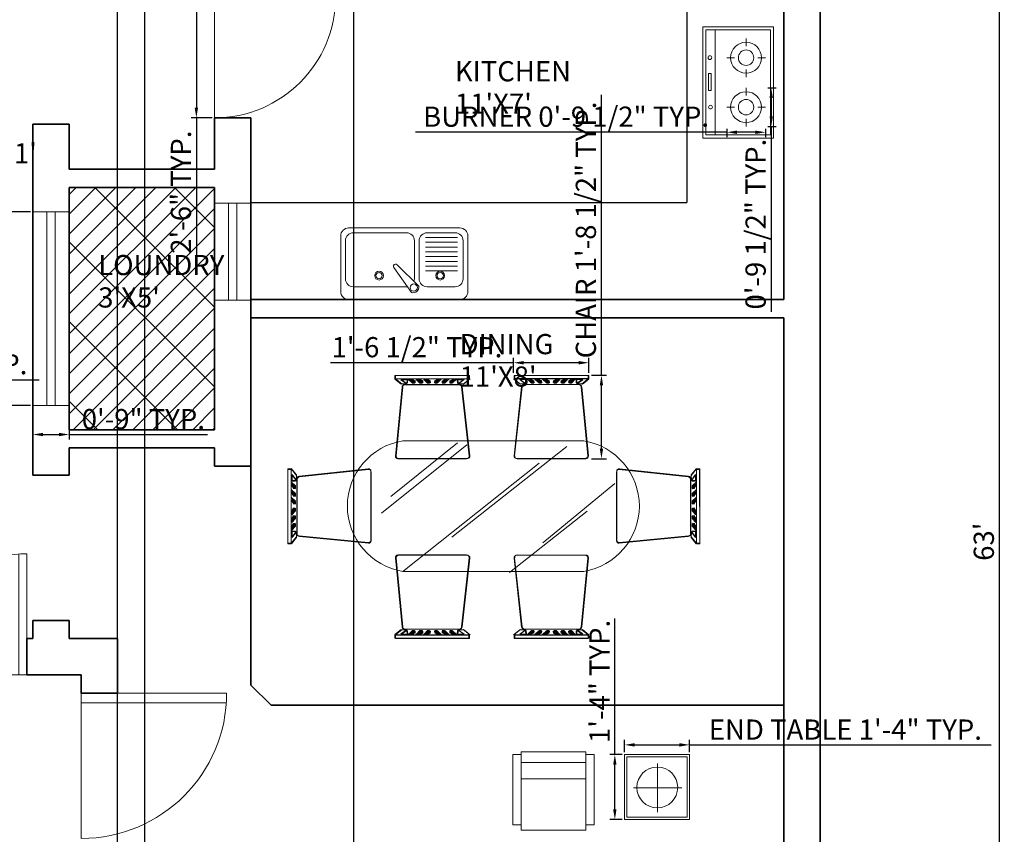
# Model space of a CAD drawing. Units: inches. Extents: x 1265 to 2734, y 1741 to 2595.
# Tile 7 of 10: x 2490 to 2734, y 2092 to 2294. Entities that reach past the tile are written whole.
import ezdxf

# ---------------------------------------------------------------- set-up
doc = ezdxf.new("R2010")
doc.units = ezdxf.units.IN
doc.header["$LTSCALE"] = 0.1
for name, color, linetype, lineweight in [('A-ANNO-DIMS', 2, 'Continuous', 18), ('A-ANNO-TEXT', 7, 'Continuous', 18), ('A-AREA-IDEN', 7, 'Continuous', 18), ('A-DOOR', 3, 'Continuous', 18), ('A-EQPM', 9, 'Continuous', 18), ('A-FLOR-CASE', 33, 'Continuous', 25), ('A-FLOR-FIXT', 9, 'Continuous', 18), ('A-FLOR-PATT', 252, 'Continuous', 13), ('A-GLAZ', 4, 'Continuous', 18), ('A-WALL', 7, 'Continuous', 35), ('C-PROP', 7, 'Continuous', 35), ('Furniture', 8, 'Continuous', 15)]:
    doc.layers.add(name, color=color, linetype=linetype, lineweight=lineweight)
doc.styles.get("Standard").update_dxf_attribs({"font": 'arial.ttf', "height": 5})
doc.dimstyles.new('ISO-25', dxfattribs={"dimtxt": 5, "dimasz": 2.5, "dimexe": 1.25, "dimexo": 0.625, "dimtad": 1, "dimlunit": 3, "dimtxsty": 'Standard', "dimcen": 2.5, "dimadec": 0, "dimazin": 0, "dimtfac": 1, "dimtmove": 0, "dimatfit": 3, "dimfxl": 1, "dimarcsym": 0})

# ---------------------------------------------------------------- blocks, each defined once
blk = doc.blocks.new('*D3')
at = {"layer": 'A-ANNO-DIMS', "color": 0, "lineweight": -2, "transparency": 16777216}
for p, q in [((2689.23, 2542.66), (2734.23, 2542.66)), ((2732.98, 2540.16), (2732.98, 1789.16)), ((2689.23, 1786.66), (2734.23, 1786.66))]:
    blk.add_line(p, q, dxfattribs=at)
at = {"layer": 'A-ANNO-DIMS', "color": 0, "lineweight": 100, "transparency": 16777216}
for points in [[(2732.56, 2540.16), (2733.39, 2540.16), (2732.98, 2542.66)], [(2732.56, 1789.16), (2733.39, 1789.16), (2732.98, 1786.66)]]:
    blk.add_solid(points, dxfattribs=at)
at = {"layer": 'Defpoints', "color": 0, "lineweight": 100, "transparency": 16777216}
for p in [(2688.6, 2542.66), (2688.6, 1786.66), (2732.98, 1786.66)]:
    blk.add_point(p, dxfattribs=at)
at = {"layer": 'A-ANNO-DIMS', "color": 0, "transparency": 16777216, "insert": (2729.8, 2164.66), "char_height": 5, "attachment_point": 5, "rotation": 90}
blk.add_mtext("63'", dxfattribs=at)
blk = doc.blocks.new('DOOR-SWING-30IN')
for p, q in [((30, 0), (30, 30)), ((0.07, 2), (30, 2)), ((0, 0), (30, 0))]:
    blk.add_line(p, q)
blk.add_arc((30, 0), 30, 90, 180)
blk = doc.blocks.new('DOOR-SWING-36IN')
for p, q in [((33.6, 35.92), (33.6, 0)), ((36, 36), (36, 0)), ((36, 0), (0, 0))]:
    blk.add_line(p, q)
blk.add_arc((36, 0), 36, 90, 180)
blk = doc.blocks.new('DOOR-PAIR-60IN')
for p, q in [((0, 30), (0, 0)), ((2, 29.93), (2, 0)), ((58, 29.93), (58, 0)), ((60, 30), (60, 0)), ((0, 0), (30, 0)), ((60, 0), (30, 0))]:
    blk.add_line(p, q)
for centre, start, end in [((0, 0), 0, 90), ((60, 0), 90, 180)]:
    blk.add_arc(centre, 30, start, end)
blk = doc.blocks.new('WINDOW-24IN')
for p, q in [((9, 24), (0, 24)), ((0, 24), (0, 0)), ((3.5, 24), (3.5, 0)), ((5.5, 24), (5.5, 0)), ((9, 24), (9, 0)), ((9, 0), (0, 0))]:
    blk.add_line(p, q)
blk = doc.blocks.new('WINDOW-48IN')
for p, q in [((0, 9), (0, 0)), ((48, 9), (0, 9)), ((48, 9), (48, 0)), ((48, 5.5), (0, 5.5)), ((48, 3.5), (0, 3.5)), ((0, 0), (48, 0))]:
    blk.add_line(p, q)
blk = doc.blocks.new('CHAIR-DINING')
for p, q in [((0.02, 0.74), (0, 17.76)), ((0.07, 0.9), (0.06, 17.92)), ((0.7, 18.39), (17.79, 16.53)), ((0.76, 18.55), (17.84, 16.69)), ((19.73, 18.48), (18.47, 16.91)), ((19.79, 18.64), (18.53, 17.07)), ((18.59, 15.75), (19.6, 17.13)), ((19.6, 17.13), (19.66, 15.62)), ((20.61, 18.35), (19.79, 18.35)), ((19.79, 18.35), (19.8, 0)), ((20.66, 18.52), (19.85, 18.52)), ((19.85, 18.52), (19.86, 0.16)), ((20.62, 0), (20.61, 18.35)), ((20.68, 0.16), (20.66, 18.52)), ((18.35, 15.9), (18.36, 2.39)), ((18.41, 16.07), (18.42, 2.55)), ((18.47, 16.91), (18.53, 15.59)), ((18.53, 17.07), (18.59, 15.75)), ((18.53, 15.59), (19.54, 16.97)), ((19.6, 15.46), (18.72, 15.52)), ((19.67, 15.09), (18.72, 14.14)), ((19.66, 15.62), (18.78, 15.69)), ((19.73, 15.25), (18.78, 14.3)), ((18.78, 13.8), (19.66, 14.74)), ((19.54, 16.97), (19.6, 15.46)), ((19.66, 14.74), (19.66, 14.37)), ((18.72, 13.64), (19.6, 14.58)), ((18.72, 14.14), (18.72, 13.64)), ((19.67, 13.2), (18.73, 12.26)), ((18.73, 11.75), (19.61, 12.7)), ((18.73, 12.26), (18.73, 11.75)), ((18.78, 14.3), (18.78, 13.8)), ((19.35, 13.64), (18.79, 13.58)), ((19.73, 13.36), (18.79, 12.42)), ((18.79, 11.92), (19.66, 12.86)), ((18.79, 12.42), (18.79, 11.92)), ((19.41, 13.8), (18.85, 13.74)), ((19.6, 14.21), (19.23, 13.76)), ((19.23, 13.76), (19.35, 13.64)), ((19.61, 12.32), (19.23, 11.88)), ((19.66, 14.37), (19.29, 13.93)), ((19.29, 13.93), (19.41, 13.8)), ((19.67, 12.48), (19.29, 12.04)), ((19.6, 14.58), (19.6, 14.21)), ((19.61, 12.7), (19.61, 12.32)), ((19.66, 12.86), (19.67, 12.48)), ((19.67, 11.31), (18.73, 10.37)), ((18.73, 9.87), (19.61, 10.81)), ((18.73, 10.37), (18.73, 9.87)), ((19.35, 11.75), (18.79, 11.69)), ((19.73, 11.48), (18.79, 10.53)), ((18.79, 10.03), (19.67, 10.97)), ((18.79, 10.53), (18.79, 10.03)), ((19.36, 9.87), (18.79, 9.8)), ((19.41, 11.92), (18.85, 11.85)), ((19.42, 10.03), (18.85, 9.97)), ((19.23, 11.88), (19.35, 11.75)), ((19.61, 10.43), (19.23, 9.99)), ((19.23, 9.99), (19.36, 9.87)), ((19.29, 12.04), (19.41, 11.92)), ((19.67, 10.6), (19.29, 10.16)), ((19.29, 10.16), (19.42, 10.03)), ((19.61, 10.81), (19.61, 10.43)), ((19.67, 10.97), (19.67, 10.6)), ((18.73, 8.11), (18.73, 8.61)), ((18.73, 8.61), (19.61, 7.67)), ((19.67, 7.17), (18.73, 8.11)), ((18.79, 8.27), (18.79, 8.77)), ((18.79, 8.77), (19.67, 7.83)), ((19.36, 8.61), (18.79, 8.67)), ((19.73, 7.33), (18.79, 8.27)), ((19.42, 8.77), (18.85, 8.84)), ((19.23, 8.48), (19.36, 8.61)), ((19.61, 8.05), (19.23, 8.48)), ((19.29, 8.65), (19.42, 8.77)), ((19.67, 8.21), (19.29, 8.65)), ((19.61, 7.67), (19.61, 8.05)), ((19.67, 7.83), (19.67, 8.21)), ((18.73, 6.22), (18.73, 6.72)), ((18.73, 6.72), (19.61, 5.78)), ((19.67, 5.28), (18.73, 6.22)), ((18.79, 6.38), (18.79, 6.89)), ((18.79, 6.89), (19.67, 5.94)), ((19.36, 6.73), (18.79, 6.79)), ((19.73, 5.44), (18.79, 6.38)), ((18.79, 4.5), (18.79, 5)), ((18.79, 5), (19.67, 4.06)), ((19.36, 4.84), (18.8, 4.9)), ((19.42, 6.89), (18.85, 6.95)), ((19.42, 5), (18.85, 5.06)), ((19.23, 6.6), (19.36, 6.73)), ((19.61, 6.16), (19.23, 6.6)), ((19.29, 6.76), (19.42, 6.89)), ((19.67, 6.32), (19.29, 6.76)), ((19.29, 4.88), (19.42, 5)), ((19.61, 5.78), (19.61, 6.16)), ((19.67, 5.94), (19.67, 6.32)), ((18.48, 1.57), (18.55, 2.89)), ((18.54, 1.73), (18.61, 3.05)), ((18.55, 2.89), (19.55, 1.51)), ((18.61, 3.05), (19.61, 1.67)), ((18.73, 4.34), (18.73, 4.84)), ((18.73, 4.84), (19.61, 3.9)), ((19.68, 3.39), (18.73, 4.34)), ((19.61, 3.02), (18.73, 2.95)), ((19.74, 3.56), (18.79, 4.5)), ((19.67, 3.18), (18.79, 3.12)), ((19.24, 4.71), (19.36, 4.84)), ((19.61, 4.27), (19.24, 4.71)), ((19.67, 4.44), (19.29, 4.88)), ((19.55, 1.51), (19.61, 3.02)), ((19.61, 3.9), (19.61, 4.27)), ((19.61, 1.67), (19.67, 3.18)), ((19.67, 4.06), (19.67, 4.44)), ((17.79, 1.77), (0.7, 0.11)), ((17.85, 1.93), (0.76, 0.27)), ((19.74, 0), (18.48, 1.57)), ((19.8, 0.16), (18.54, 1.73)), ((19.8, 0), (20.62, 0)), ((19.86, 0.16), (20.68, 0.16))]:
    blk.add_line(p, q)
for centre, start, end in [((0.63, 17.76), 83.7931, 180.0502), ((0.69, 17.92), 83.7931, 180.0502), ((17.72, 15.9), 0.0502, 83.7931), ((17.78, 16.06), 0.0502, 83.7931), ((17.79, 2.55), 275.5303, 0.0502), ((0.64, 0.74), 180.0502, 275.5303), ((0.7, 0.9), 180.0502, 275.5303), ((17.73, 2.39), 275.5303, 0.0502)]:
    blk.add_arc(centre, 0.629, start, end)
blk = doc.blocks.new('END-TABLE-ROUND-LAMP')
for p, q in [((0, 0), (0, 16.08)), ((0, 16.08), (16.08, 16.08)), ((0.58, 0.59), (0.58, 15.5)), ((0.58, 15.5), (15.49, 15.5)), ((15.49, 15.5), (15.49, 0.59)), ((16.08, 16.08), (16.08, 0)), ((8.18, 13.85), (8.18, 1.8)), ((14.2, 7.89), (2.22, 7.89)), ((16.08, 0), (0, 0)), ((15.49, 0.59), (0.58, 0.59))]:
    blk.add_line(p, q)
blk.add_circle((8.11, 7.95), 5.06)
blk = doc.blocks.new('COOKTOP-BURNER')
for p, q in [((4.79, 9.57), (4.79, 7.66)), ((1.91, 4.79), (0, 4.79)), ((9.57, 4.79), (7.66, 4.79)), ((4.79, 1.91), (4.79, 0))]:
    blk.add_line(p, q)
for radius in [3.83, 1.91]:
    blk.add_circle((4.79, 4.79), radius)
blk = doc.blocks.new('*D25')
at = {"layer": 'A-ANNO-DIMS', "color": 0, "lineweight": -2, "transparency": 16777216}
for p, q in [((2537.98, 2299.66), (2532.85, 2299.66)), ((2534.1, 2297.16), (2534.1, 2272.16)), ((2537.98, 2269.66), (2532.85, 2269.66)), ((2534.1, 2269.66), (2534.1, 2235.34))]:
    blk.add_line(p, q, dxfattribs=at)
at = {"layer": 'A-ANNO-DIMS', "color": 0, "lineweight": 100, "transparency": 16777216}
for points in [[(2533.69, 2297.16), (2534.52, 2297.16), (2534.1, 2299.66)], [(2533.69, 2272.16), (2534.52, 2272.16), (2534.1, 2269.66)]]:
    blk.add_solid(points, dxfattribs=at)
at = {"layer": 'Defpoints', "color": 0, "lineweight": 100, "transparency": 16777216}
for p in [(2538.6, 2299.66), (2534.1, 2269.66), (2538.6, 2269.66)]:
    blk.add_point(p, dxfattribs=at)
at = {"layer": 'A-ANNO-DIMS', "color": 0, "transparency": 16777216, "insert": (2530.92, 2251.25), "char_height": 5, "attachment_point": 5, "rotation": 90}
blk.add_mtext('2\'-6" TYP.', dxfattribs=at)
blk = doc.blocks.new('*D28')
at = {"layer": 'A-ANNO-DIMS', "color": 0, "lineweight": -2, "transparency": 16777216}
for p, q in [((2665.48, 2266.09), (2588.38, 2266.09)), ((2665.48, 2266.9), (2665.48, 2264.84)), ((2672.55, 2266.09), (2667.98, 2266.09)), ((2675.05, 2266.9), (2675.05, 2264.84))]:
    blk.add_line(p, q, dxfattribs=at)
at = {"layer": 'A-ANNO-DIMS', "color": 0, "lineweight": 100, "transparency": 16777216}
for points in [[(2667.98, 2266.5), (2667.98, 2265.67), (2665.48, 2266.09)], [(2672.55, 2266.5), (2672.55, 2265.67), (2675.05, 2266.09)]]:
    blk.add_solid(points, dxfattribs=at)
at = {"layer": 'Defpoints', "color": 0, "lineweight": 100, "transparency": 16777216}
for p in [(2665.48, 2267.52), (2665.48, 2266.09), (2675.05, 2267.52)]:
    blk.add_point(p, dxfattribs=at)
at = {"layer": 'A-ANNO-DIMS', "color": 0, "transparency": 16777216, "insert": (2625.68, 2269.3), "char_height": 5, "attachment_point": 5}
blk.add_mtext('BURNER 0\'-9 1/2" TYP.', dxfattribs=at)
blk = doc.blocks.new('*D29')
at = {"layer": 'A-ANNO-DIMS', "color": 0, "lineweight": -2, "transparency": 16777216}
for p, q in [((2675.67, 2277.09), (2677.73, 2277.09)), ((2676.48, 2274.59), (2676.48, 2270.02)), ((2675.67, 2267.52), (2677.73, 2267.52)), ((2676.48, 2267.52), (2676.48, 2221.64))]:
    blk.add_line(p, q, dxfattribs=at)
at = {"layer": 'A-ANNO-DIMS', "color": 0, "lineweight": 100, "transparency": 16777216}
for points in [[(2676.07, 2274.59), (2676.9, 2274.59), (2676.48, 2277.09)], [(2676.07, 2270.02), (2676.9, 2270.02), (2676.48, 2267.52)]]:
    blk.add_solid(points, dxfattribs=at)
at = {"layer": 'Defpoints', "color": 0, "lineweight": 100, "transparency": 16777216}
for p in [(2675.05, 2277.09), (2675.05, 2267.52), (2676.48, 2267.52)]:
    blk.add_point(p, dxfattribs=at)
at = {"layer": 'A-ANNO-DIMS', "color": 0, "transparency": 16777216, "insert": (2673.27, 2243.33), "char_height": 5, "attachment_point": 5, "rotation": 90}
blk.add_mtext('0\'-9 1/2" TYP.', dxfattribs=at)
blk = doc.blocks.new('*D30')
at = {"layer": 'A-ANNO-DIMS', "color": 0, "lineweight": -2, "transparency": 16777216}
for p, q in [((2634.44, 2205.89), (2634.44, 2275.38)), ((2631.96, 2205.89), (2635.69, 2205.89)), ((2634.44, 2187.71), (2634.44, 2203.39)), ((2631.96, 2185.21), (2635.69, 2185.21))]:
    blk.add_line(p, q, dxfattribs=at)
at = {"layer": 'A-ANNO-DIMS', "color": 0, "lineweight": 100, "transparency": 16777216}
for points in [[(2634.02, 2203.39), (2634.85, 2203.39), (2634.44, 2205.89)], [(2634.02, 2187.71), (2634.85, 2187.71), (2634.44, 2185.21)]]:
    blk.add_solid(points, dxfattribs=at)
at = {"layer": 'Defpoints', "color": 0, "lineweight": 100, "transparency": 16777216}
for p in [(2631.33, 2205.89), (2634.44, 2205.89), (2631.33, 2185.21)]:
    blk.add_point(p, dxfattribs=at)
at = {"layer": 'A-ANNO-DIMS', "color": 0, "transparency": 16777216, "insert": (2631.23, 2241.88), "char_height": 5, "attachment_point": 5, "rotation": 90}
blk.add_mtext('CHAIR 1\'-8 1/2" TYP.', dxfattribs=at)
blk = doc.blocks.new('*D31')
at = {"layer": 'A-ANNO-DIMS', "color": 0, "lineweight": -2, "transparency": 16777216}
for p, q in [((2612.69, 2206.51), (2612.69, 2210.24)), ((2631.33, 2206.51), (2631.33, 2210.24)), ((2612.69, 2208.99), (2567.29, 2208.99)), ((2628.83, 2208.99), (2615.19, 2208.99))]:
    blk.add_line(p, q, dxfattribs=at)
at = {"layer": 'A-ANNO-DIMS', "color": 0, "lineweight": 100, "transparency": 16777216}
for points in [[(2615.19, 2209.41), (2615.19, 2208.57), (2612.69, 2208.99)], [(2628.83, 2209.41), (2628.83, 2208.57), (2631.33, 2208.99)]]:
    blk.add_solid(points, dxfattribs=at)
at = {"layer": 'Defpoints', "color": 0, "lineweight": 100, "transparency": 16777216}
for p in [(2612.69, 2208.99), (2612.69, 2205.89), (2631.33, 2205.89)]:
    blk.add_point(p, dxfattribs=at)
at = {"layer": 'A-ANNO-DIMS', "color": 0, "transparency": 16777216, "insert": (2588.74, 2212.2), "char_height": 5, "attachment_point": 5}
blk.add_mtext('1\'-6 1/2" TYP.', dxfattribs=at)
blk = doc.blocks.new('*D32')
at = {"layer": 'A-ANNO-DIMS', "color": 0, "lineweight": -2, "transparency": 16777216}
for p, q in [((2369.76, 2201.71), (2369.76, 2206.02)), ((2372.26, 2204.77), (2391.87, 2204.77)), ((2394.37, 2201.71), (2394.37, 2206.02)), ((2394.37, 2204.77), (2495.13, 2204.77))]:
    blk.add_line(p, q, dxfattribs=at)
at = {"layer": 'A-ANNO-DIMS', "color": 0, "lineweight": 100, "transparency": 16777216}
for points in [[(2372.26, 2205.19), (2372.26, 2204.36), (2369.76, 2204.77)], [(2391.87, 2205.19), (2391.87, 2204.36), (2394.37, 2204.77)]]:
    blk.add_solid(points, dxfattribs=at)
at = {"layer": 'Defpoints', "color": 0, "lineweight": 100, "transparency": 16777216}
for p in [(2394.37, 2204.77), (2369.76, 2201.08), (2394.37, 2201.08)]:
    blk.add_point(p, dxfattribs=at)
at = {"layer": 'A-ANNO-DIMS', "color": 0, "transparency": 16777216, "insert": (2446, 2207.99), "char_height": 5, "attachment_point": 5}
blk.add_mtext('LOUNGE CHAIR 2\'-0 1/2" TYP.', dxfattribs=at)
blk = doc.blocks.new('*D36')
at = {"layer": 'A-ANNO-DIMS', "color": 0, "lineweight": -2, "transparency": 16777216}
for p, q in [((2492.98, 2246.41), (2485.15, 2246.41)), ((2486.4, 2243.91), (2486.4, 2200.91)), ((2492.98, 2198.41), (2485.15, 2198.41)), ((2486.4, 2198.41), (2486.4, 2131.39))]:
    blk.add_line(p, q, dxfattribs=at)
at = {"layer": 'A-ANNO-DIMS', "color": 0, "lineweight": 100, "transparency": 16777216}
for points in [[(2485.99, 2243.91), (2486.82, 2243.91), (2486.4, 2246.41)], [(2485.99, 2200.91), (2486.82, 2200.91), (2486.4, 2198.41)]]:
    blk.add_solid(points, dxfattribs=at)
at = {"layer": 'Defpoints', "color": 0, "lineweight": 100, "transparency": 16777216}
for p in [(2493.6, 2246.41), (2486.4, 2198.41), (2493.6, 2198.41)]:
    blk.add_point(p, dxfattribs=at)
at = {"layer": 'A-ANNO-DIMS', "color": 0, "transparency": 16777216, "insert": (2483.19, 2163.65), "char_height": 5, "attachment_point": 5, "rotation": 90}
blk.add_mtext('WINDOW 4\'-0" TYP.', dxfattribs=at)
blk = doc.blocks.new('*D37')
at = {"layer": 'A-ANNO-DIMS', "color": 0, "lineweight": -2, "transparency": 16777216}
for p, q in [((2493.6, 2197.78), (2493.6, 2189.96)), ((2502.6, 2197.78), (2502.6, 2189.96)), ((2496.1, 2191.21), (2500.1, 2191.21)), ((2502.6, 2191.21), (2536.83, 2191.21))]:
    blk.add_line(p, q, dxfattribs=at)
at = {"layer": 'A-ANNO-DIMS', "color": 0, "lineweight": 100, "transparency": 16777216}
for points in [[(2496.1, 2191.62), (2496.1, 2190.79), (2493.6, 2191.21)], [(2500.1, 2191.62), (2500.1, 2190.79), (2502.6, 2191.21)]]:
    blk.add_solid(points, dxfattribs=at)
at = {"layer": 'Defpoints', "color": 0, "lineweight": 100, "transparency": 16777216}
for p in [(2493.6, 2198.41), (2502.6, 2198.41), (2502.6, 2191.21)]:
    blk.add_point(p, dxfattribs=at)
at = {"layer": 'A-ANNO-DIMS', "color": 0, "transparency": 16777216, "insert": (2520.97, 2194.38), "char_height": 5, "attachment_point": 5}
blk.add_mtext('0\'-9" TYP.', dxfattribs=at)
blk = doc.blocks.new('*D38')
at = {"layer": 'A-ANNO-DIMS', "color": 0, "lineweight": -2, "transparency": 16777216}
for p, q in [((2640.17, 2112.54), (2640.17, 2115.58)), ((2656.25, 2112.54), (2656.25, 2115.58)), ((2642.67, 2114.33), (2653.75, 2114.33)), ((2656.25, 2114.33), (2730.97, 2114.33))]:
    blk.add_line(p, q, dxfattribs=at)
at = {"layer": 'A-ANNO-DIMS', "color": 0, "lineweight": 100, "transparency": 16777216}
for points in [[(2642.67, 2114.75), (2642.67, 2113.91), (2640.17, 2114.33)], [(2653.75, 2114.75), (2653.75, 2113.91), (2656.25, 2114.33)]]:
    blk.add_solid(points, dxfattribs=at)
at = {"layer": 'Defpoints', "color": 0, "lineweight": 100, "transparency": 16777216}
for p in [(2656.25, 2114.33), (2640.17, 2111.92), (2656.25, 2111.92)]:
    blk.add_point(p, dxfattribs=at)
at = {"layer": 'A-ANNO-DIMS', "color": 0, "transparency": 16777216, "insert": (2694.86, 2117.47), "char_height": 5, "attachment_point": 5}
blk.add_mtext('END TABLE 1\'-4" TYP.', dxfattribs=at)
blk = doc.blocks.new('*D39')
at = {"layer": 'A-ANNO-DIMS', "color": 0, "lineweight": -2, "transparency": 16777216}
for p, q in [((2637.76, 2111.92), (2637.76, 2145.67)), ((2639.54, 2111.92), (2636.51, 2111.92)), ((2637.76, 2098.34), (2637.76, 2109.42)), ((2639.54, 2095.84), (2636.51, 2095.84))]:
    blk.add_line(p, q, dxfattribs=at)
at = {"layer": 'A-ANNO-DIMS', "color": 0, "lineweight": 100, "transparency": 16777216}
for points in [[(2637.34, 2109.42), (2638.17, 2109.42), (2637.76, 2111.92)], [(2637.34, 2098.34), (2638.17, 2098.34), (2637.76, 2095.84)]]:
    blk.add_solid(points, dxfattribs=at)
at = {"layer": 'Defpoints', "color": 0, "lineweight": 100, "transparency": 16777216}
for p in [(2637.76, 2111.92), (2640.17, 2111.92), (2640.17, 2095.84)]:
    blk.add_point(p, dxfattribs=at)
at = {"layer": 'A-ANNO-DIMS', "color": 0, "transparency": 16777216, "insert": (2634.62, 2130.05), "char_height": 5, "attachment_point": 5, "rotation": 90}
blk.add_mtext('1\'-4" TYP.', dxfattribs=at)
blk = doc.blocks.new('*D42')
at = {"layer": 'A-ANNO-DIMS', "color": 0, "lineweight": -2, "transparency": 16777216}
for p, q in [((2328.6, 1822.68), (2328.6, 2585.16)), ((2331.1, 2583.91), (2518.82, 2583.91)), ((2521.32, 1822.68), (2521.32, 2585.16))]:
    blk.add_line(p, q, dxfattribs=at)
at = {"layer": 'A-ANNO-DIMS', "color": 0, "lineweight": 100, "transparency": 16777216}
for points in [[(2331.1, 2584.32), (2331.1, 2583.49), (2328.6, 2583.91)], [(2518.82, 2584.32), (2518.82, 2583.49), (2521.32, 2583.91)]]:
    blk.add_solid(points, dxfattribs=at)
at = {"layer": 'Defpoints', "color": 0, "lineweight": 100, "transparency": 16777216}
for p in [(2521.32, 2583.91), (2328.6, 1822.06), (2521.32, 1822.06)]:
    blk.add_point(p, dxfattribs=at)
at = {"layer": 'A-ANNO-DIMS', "color": 0, "transparency": 16777216, "insert": (2424.96, 2587.12), "char_height": 5, "attachment_point": 5}
blk.add_mtext('16\'-0 1/2"', dxfattribs=at)
blk = doc.blocks.new('*D47')
at = {"layer": 'A-ANNO-DIMS', "color": 0, "lineweight": -2, "transparency": 16777216}
for p, q in [((2514.6, 1992.78), (2514.6, 2585.16)), ((2517.1, 2583.91), (2570.6, 2583.91)), ((2573.1, 1992.78), (2573.1, 2585.16))]:
    blk.add_line(p, q, dxfattribs=at)
at = {"layer": 'A-ANNO-DIMS', "color": 0, "lineweight": 100, "transparency": 16777216}
for points in [[(2517.1, 2584.32), (2517.1, 2583.49), (2514.6, 2583.91)], [(2570.6, 2584.32), (2570.6, 2583.49), (2573.1, 2583.91)]]:
    blk.add_solid(points, dxfattribs=at)
at = {"layer": 'Defpoints', "color": 0, "lineweight": 100, "transparency": 16777216}
for p in [(2573.1, 2583.91), (2514.6, 1992.16), (2573.1, 1992.16)]:
    blk.add_point(p, dxfattribs=at)
at = {"layer": 'A-ANNO-DIMS', "color": 0, "transparency": 16777216, "insert": (2543.85, 2587.12), "char_height": 5, "attachment_point": 5}
blk.add_mtext('4\'-10 1/2"', dxfattribs=at)

msp = doc.modelspace()

# ---------------------------------------------------------------- hatches: boundary and pattern name
at = {"layer": 'A-FLOR-PATT'}
h = msp.add_hatch(dxfattribs=at)
h.set_pattern_fill('GRATE', color=256, scale=4.4, angle=45)
h.paths.add_polyline_path([(2538.602, 2252.407), (2502.602, 2252.407), (2502.602, 2192.407), (2538.602, 2192.407)])

# ---------------------------------------------------------------- linework, layer by layer
at = {"layer": 'A-EQPM'}
for p, q in [((2677.04, 2292.207), (2659.541, 2292.207)), ((2659.541, 2292.207), (2659.541, 2264.651)), ((2676.275, 2291.442), (2660.306, 2291.442)), ((2660.306, 2291.442), (2660.306, 2265.417)), ((2662.603, 2291.442), (2662.603, 2265.417)), ((2676.275, 2291.442), (2676.275, 2265.417)), ((2677.04, 2292.207), (2677.04, 2264.651)), ((2660.977, 2276.435), (2660.977, 2280.656)), ((2660.977, 2280.656), (2661.585, 2280.656)), ((2661.585, 2280.656), (2661.585, 2276.435)), ((2661.585, 2276.435), (2660.977, 2276.435)), ((2677.04, 2264.651), (2659.541, 2264.651)), ((2676.275, 2265.417), (2660.306, 2265.417))]:
    msp.add_line(p, q, dxfattribs=at)
for centre in [(2661.315, 2284.572), (2661.45, 2272.316)]:
    msp.add_circle(centre, 0.459, dxfattribs=at)
at = {"layer": 'A-FLOR-CASE'}
for p in [(2655.602, 2308.657), (2547.602, 2248.657)]:
    msp.add_line(p, (2655.602, 2248.657), dxfattribs=at)
at = {"layer": 'A-FLOR-FIXT'}
for p, q in [((2599.38, 2242.373), (2571.821, 2242.373)), ((2569.852, 2240.405), (2569.852, 2226.625)), ((2571.033, 2239.224), (2571.033, 2229.775)), ((2586.14, 2241.192), (2573.002, 2241.192)), ((2588.108, 2229.775), (2588.108, 2239.224)), ((2589.289, 2229.775), (2589.289, 2239.224)), ((2590.873, 2240.018), (2598.761, 2240.018)), ((2598.199, 2241.192), (2591.258, 2241.192)), ((2600.167, 2229.775), (2600.167, 2239.224)), ((2601.348, 2226.625), (2601.348, 2240.405)), ((2590.873, 2238.836), (2598.761, 2238.836)), ((2590.873, 2237.655), (2598.761, 2237.655)), ((2590.873, 2236.474), (2598.761, 2236.474)), ((2590.873, 2235.293), (2598.761, 2235.293)), ((2590.873, 2234.112), (2598.761, 2234.112)), ((2587.406, 2226.422), (2583.018, 2232.557)), ((2589.202, 2227.958), (2583.824, 2233.247)), ((2590.873, 2232.931), (2598.761, 2232.931)), ((2590.873, 2231.75), (2598.761, 2231.75)), ((2573.002, 2227.806), (2586.14, 2227.806)), ((2598.199, 2227.806), (2591.258, 2227.806)), ((2571.821, 2224.657), (2599.38, 2224.657))]:
    msp.add_line(p, q, dxfattribs=at)
for centre, radius in [((2579.355, 2230.568), 1.081), ((2594.501, 2230.568), 1.081), ((2579.355, 2230.568), 0.788), ((2594.501, 2230.568), 0.788), ((2587.946, 2227.609), 0.892)]:
    msp.add_circle(centre, radius, dxfattribs=at)
for centre, radius, start, end in [((2571.821, 2240.405), 1.968, 90, 180), ((2599.38, 2240.405), 1.968, 0, 90), ((2573.002, 2239.224), 1.968, 90, 180), ((2586.14, 2239.224), 1.968, 0, 90), ((2591.258, 2239.224), 1.968, 90, 180), ((2598.199, 2239.224), 1.968, 0, 90), ((2583.416, 2232.908), 0.531, 39.73777, 221.31634), ((2573.002, 2229.775), 1.968, 180, 270), ((2586.14, 2229.775), 1.968, 341.10956, 0), ((2591.258, 2229.775), 1.968, 180, 270), ((2598.199, 2229.775), 1.968, 270, 0), ((2586.14, 2229.775), 1.968, 270, 277.6978), ((2587.861, 2227.708), 1.364, 250.52706, 10.52706), ((2571.821, 2226.625), 1.968, 180, 270), ((2599.38, 2226.625), 1.968, 270, 0)]:
    msp.add_arc(centre, radius, start, end, dxfattribs=at)
at = {"layer": 'A-WALL'}
for p, q in [((2679.602, 2308.657), (2679.602, 2224.657)), ((2538.602, 2269.657), (2538.602, 2256.907)), ((2538.602, 2269.657), (2547.602, 2269.657)), ((2547.602, 2269.657), (2547.602, 2129.157)), ((2547.602, 2269.657), (2547.602, 2224.657)), ((2493.602, 2181.157), (2493.602, 2268.13)), ((2493.602, 2268.13), (2502.602, 2268.13)), ((2502.602, 2256.907), (2502.602, 2268.13)), ((2538.602, 2256.907), (2502.602, 2256.907)), ((2502.602, 2192.407), (2502.602, 2252.407)), ((2538.602, 2252.407), (2502.602, 2252.407)), ((2538.602, 2252.407), (2538.602, 2192.407)), ((2547.602, 2224.657), (2679.602, 2224.657)), ((2547.602, 2220.157), (2679.602, 2220.157)), ((2547.602, 2220.157), (2547.602, 2183.407)), ((2679.602, 2220.157), (2679.602, 1992.157)), ((2538.602, 2192.407), (2502.602, 2192.407)), ((2538.602, 2187.907), (2502.602, 2187.907)), ((2502.602, 2181.157), (2502.602, 2187.907)), ((2538.602, 2187.907), (2538.602, 2183.407)), ((2547.602, 2183.407), (2538.602, 2183.407)), ((2493.602, 2181.157), (2502.602, 2181.157)), ((2493.602, 2140.657), (2493.602, 2145.157)), ((2493.602, 2145.157), (2502.602, 2145.157)), ((2502.602, 2140.657), (2502.602, 2145.157)), ((2492.143, 2140.657), (2492.143, 2131.657)), ((2492.143, 2140.657), (2493.602, 2140.657)), ((2502.602, 2140.657), (2514.602, 2140.657)), ((2514.602, 2127.157), (2514.602, 2140.657)), ((2492.143, 2131.657), (2505.602, 2131.657)), ((2505.602, 2127.157), (2505.602, 2131.657)), ((2547.602, 2129.157), (2552.602, 2124.157)), ((2505.602, 2127.157), (2514.602, 2127.157)), ((2552.602, 2124.157), (2679.602, 2124.157))]:
    msp.add_line(p, q, dxfattribs=at)
at = {"layer": 'C-PROP'}
msp.add_line((2688.602, 2542.657), (2688.602, 1786.657), dxfattribs=at)
at = {"layer": 'Furniture'}
for p, q in [((2579.982, 2171.734, 3.573), (2601.085, 2188.688, 3.573)), ((2582.276, 2175.858, 3.573), (2598.791, 2189.146, 3.573)), ((2630.046, 2189.658, 3.573), (2585.283, 2189.658, 3.573)), ((2597.415, 2165.777, 3.573), (2625.858, 2188.229, 3.573)), ((2585.283, 2157.315, 3.573), (2618.977, 2184.105, 3.573)), ((2619.894, 2164.402, 3.573), (2637.786, 2179.065, 3.573)), ((2611.637, 2157.071, 3.573), (2630.905, 2172.192, 3.573)), ((2585.283, 2157.315, 3.573), (2630.046, 2157.315, 3.573)), ((2630.6, 2112.626), (2614.521, 2112.626)), ((2614.521, 2112.626), (2614.521, 2093.197)), ((2630.6, 2093.197), (2630.6, 2112.626)), ((2614.521, 2111.956), (2612.511, 2111.956)), ((2612.511, 2111.956), (2612.511, 2094.537)), ((2630.6, 2109.946), (2614.521, 2109.946)), ((2632.61, 2111.956), (2630.6, 2111.956)), ((2632.61, 2094.537), (2632.61, 2111.956)), ((2614.521, 2105.926), (2630.6, 2105.926)), ((2612.511, 2094.537), (2614.521, 2094.537)), ((2614.521, 2093.197), (2630.6, 2093.197)), ((2630.6, 2094.537), (2632.61, 2094.537))]:
    msp.add_line(p, q, dxfattribs=at)
for centre, start, end in [((2587.883, 2173.486, 3.573), 99.13208, 260.86792), ((2627.447, 2173.486, 3.573), 279.13208, 80.86792)]:
    msp.add_arc(centre, 16.379, start, end, dxfattribs=at)

# ---------------------------------------------------------------- block references
at = {"layer": 'A-DOOR', "rotation": 180}
msp.add_blockref('DOOR-SWING-30IN', (2568.603, 2299.656), dxfattribs=at)
at = {"layer": 'A-DOOR'}
msp.add_blockref('DOOR-PAIR-60IN', (2432.143, 2131.657), dxfattribs=at)
at = {"layer": 'A-DOOR', "extrusion": (0, 0, -1), "zscale": -1, "rotation": 90.0000000000019}
msp.add_blockref('DOOR-SWING-36IN', (-2505.603, 2091.156), dxfattribs=at)
at = {"layer": 'A-EQPM'}
msp.add_blockref('COOKTOP-BURNER', (2665.476, 2279.765), dxfattribs=at)
at = {"layer": 'A-EQPM', "rotation": 180}
msp.add_blockref('COOKTOP-BURNER', (2675.047, 2277.093), dxfattribs=at)
at = {"layer": 'A-GLAZ'}
for name, p, rotation in [('WINDOW-48IN', (2493.603, 2246.407), 269.9999999999986), ('WINDOW-24IN', (2547.603, 2248.491), 180)]:
    msp.add_blockref(name, p, dxfattribs=dict(at, rotation=rotation))
at = {"layer": 'Furniture', "extrusion": (0, 0, -1), "zscale": -1}
for p, rotation in [((-2583.293, 2185.186), 89.94977784564419), ((-2631.335, 2161.367), 269.9999999999911)]:
    msp.add_blockref('CHAIR-DINING', p, dxfattribs=dict(at, rotation=rotation))
at = {"layer": 'Furniture'}
for p, rotation in [((2631.335, 2185.207), 90.00000000000269), ((2583.293, 2161.388), 269.9497778456416)]:
    msp.add_blockref('CHAIR-DINING', p, dxfattribs=dict(at, rotation=rotation))
at = {"layer": 'Furniture', "extrusion": (0, 0, -1), "zscale": -1}
msp.add_blockref('CHAIR-DINING', (-2577.408, 2164.167), dxfattribs=at)
at = {"layer": 'Furniture'}
for name, p in [('CHAIR-DINING', (2638.158, 2164.167)), ('END-TABLE-ROUND-LAMP', (2640.17, 2095.837))]:
    msp.add_blockref(name, p, dxfattribs=at)

# ---------------------------------------------------------------- texts
at = {"layer": 'A-ANNO-TEXT'}
msp.add_text("CELLING HEIGHT-11'", height=5, dxfattribs=at).set_placement((2429.091, 2258.376))
at = {"layer": 'A-AREA-IDEN'}
for s, p in [('KITCHEN', (2598.14, 2278.699)), ("11'X7'", (2598.14, 2270.667)), ('LOUNDRY', (2509.786, 2230.691)), ("3'X5'", (2509.786, 2222.659)), ('DINING', (2599.32, 2211.105)), ("11'X8'", (2599.32, 2203.073))]:
    msp.add_text(s, height=5, dxfattribs=at).set_placement(p)

# ---------------------------------------------------------------- dimensions: what is measured, and where the dimension line sits
at = {"layer": 'A-ANNO-DIMS'}
for base, p1, p2, picture, middle in [((2521.319, 2583.907), (2328.602, 1822.059), (2521.319, 1822.059), '*D42', (2424.961, 2587.117)), ((2573.102, 2583.907), (2514.602, 1992.157), (2573.102, 1992.157), '*D47', (2543.852, 2587.117))]:
    dim = msp.add_linear_dim(base=base, p1=p1, p2=p2, dimstyle='ISO-25', override={"dimdec": 1, "dimlfac": 1, "dimrnd": 0, "dimzin": 1, "dimdsep": 46, "dimlunit": 4, "dimfrac": 2}, dxfattribs=at)
    dim.commit()
    dim.dimension.update_dxf_attribs({"geometry": picture, "text_midpoint": middle})
dim = msp.add_linear_dim(base=(2732.978, 1786.657), p1=(2688.602, 2542.657), p2=(2688.602, 1786.657), angle=90, dimstyle='ISO-25', override={"dimclrd": 0, "dimclre": 0, "dimclrt": 0}, dxfattribs=at)
dim.commit()
dim.dimension.update_dxf_attribs({"geometry": '*D3', "text_midpoint": (2729.798, 2164.657)})
for base, p1, p2, angle, text, picture, middle in [((2534.102, 2269.657), (2538.602, 2299.657), (2538.602, 2269.657), 270, '<> TYP.', '*D25', (2530.925, 2251.25)), ((2665.476, 2266.087), (2675.047, 2267.522), (2665.476, 2267.522), 180, 'BURNER <> TYP.', '*D28', (2625.68, 2269.297)), ((2676.482, 2267.522), (2675.047, 2277.093), (2675.047, 2267.522), 270, '<> TYP.', '*D29', (2673.272, 2243.333)), ((2634.437, 2205.888), (2631.335, 2185.207), (2631.335, 2205.888), 90, 'CHAIR <> TYP.', '*D30', (2631.227, 2241.885)), ((2486.402, 2198.407), (2493.602, 2246.407), (2493.602, 2198.407), 270, 'WINDOW <> TYP.', '*D36', (2483.19, 2163.646)), ((2612.694, 2208.99), (2631.335, 2205.888), (2612.694, 2205.888), 180, '<> TYP.', '*D31', (2588.74, 2212.2)), ((2637.758, 2111.917), (2640.17, 2095.837), (2640.17, 2111.917), 90, '<> TYP.', '*D39', (2634.621, 2130.045))]:
    dim = msp.add_linear_dim(base=base, p1=p1, p2=p2, angle=angle, text=text, dimstyle='ISO-25', override={"dimdec": 1, "dimlfac": 1, "dimrnd": 0, "dimzin": 1, "dimdsep": 46, "dimlunit": 4, "dimfrac": 2}, dxfattribs=at)
    dim.commit()
    dim.dimension.update_dxf_attribs({"geometry": picture, "text_midpoint": middle})
for base, p1, p2, text, picture, middle in [((2394.366, 2204.774), (2369.755, 2201.083), (2394.366, 2201.083), 'LOUNGE CHAIR <> TYP.', '*D32', (2446, 2207.986)), ((2502.602, 2191.207), (2493.602, 2198.407), (2502.602, 2198.407), '<> TYP.', '*D37', (2520.966, 2194.385)), ((2656.249, 2114.329), (2640.17, 2111.917), (2656.249, 2111.917), 'END TABLE <> TYP.', '*D38', (2694.86, 2117.466))]:
    dim = msp.add_linear_dim(base=base, p1=p1, p2=p2, text=text, dimstyle='ISO-25', override={"dimdec": 1, "dimlfac": 1, "dimrnd": 0, "dimzin": 1, "dimdsep": 46, "dimlunit": 4, "dimfrac": 2}, dxfattribs=at)
    dim.commit()
    dim.dimension.update_dxf_attribs({"geometry": picture, "text_midpoint": middle})

doc.saveas('drawing.dxf')
